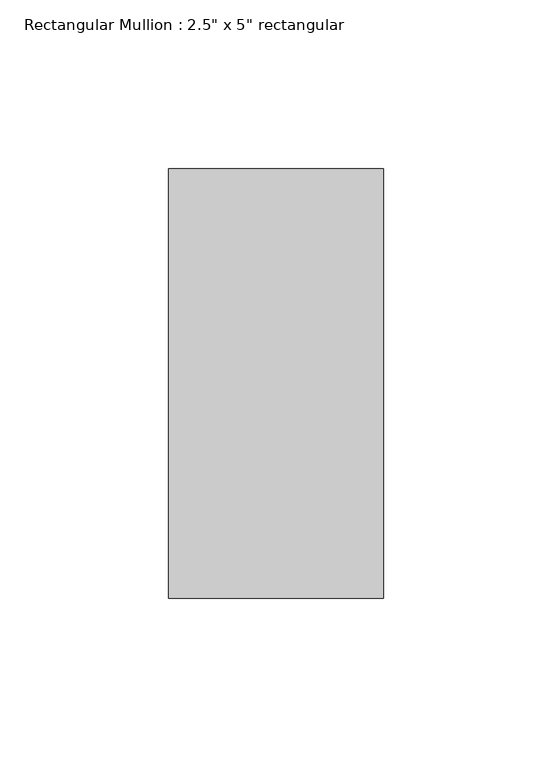
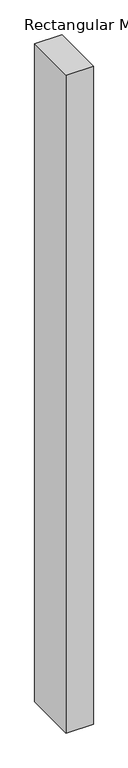
"""IFC4 building model written with IfcOpenShell, lengths in millimetres: member geometry."""

from ifc_helpers import new_model, si_unit, frame, origin, place, context, project, spatial, polyline, outline, extrude, source, transform, mapped, element, save


def member_d1d39edc(model_context):
    return source(origin(), model_context, "Body", "SweptSolid", [
        extrude(outline(polyline([(0.0, 63.5), (0.0, -63.5), (-63.5, -63.5), (-63.5, 63.5), (0.0, 63.5)])), frame((0.0, 0.0, -1624.1102394), z_axis=(0.0, 0.0, 1.0), x_axis=(1.0, 0.0, 0.0)), (0.0, 0.0, 1.0), 1624.1102394),
    ])


if __name__ == "__main__":
    model = new_model("IFC4")
    model_context = context("Model", 3, world=origin())
    ifc_project = project(units=[si_unit("LENGTHUNIT", "METRE", prefix="MILLI")], contexts=[model_context])
    site = spatial("IfcSite", under=ifc_project)
    building = spatial("IfcBuilding", under=site)
    placement = place(None, origin())
    member_shape = member_d1d39edc(model_context)
    element("IfcMember", 1, ObjectType="Rectangular Mullion : 2.5\" x 5\" rectangular", at=placement, inside=building, context=model_context, shape_type="MappedRepresentation", body=[
        mapped(member_shape, transform((0.0, 0.0, 0.0), x_axis=(1.0, 0.0, 0.0), y_axis=(0.0, 1.0, 0.0), z_axis=(0.0, 0.0, 1.0))),
    ])
    save(model, "model.ifc")

# Revit data of these elements
# Type "Rectangular Mullion : 2.5\" x 5\" rectangular"
#   built-in parameter 1007304 = 0.416667 (stored number, unit not read)
#   built-in parameter 1007301 = 0.104167 (stored number, unit not read)
#   built-in parameter 1007300 = 0.104167 (stored number, unit not read)
# Element 1 (IfcMember, "Rectangular Mullion : 2.5\" x 5\" rectangular")
#   Materials on its faces: "Aluminum"
# Materials
#   "Aluminum": class "Metal", colour RGB 247 247 247, transparency 0, Description = "Aluminum 6061", Cost = 0
